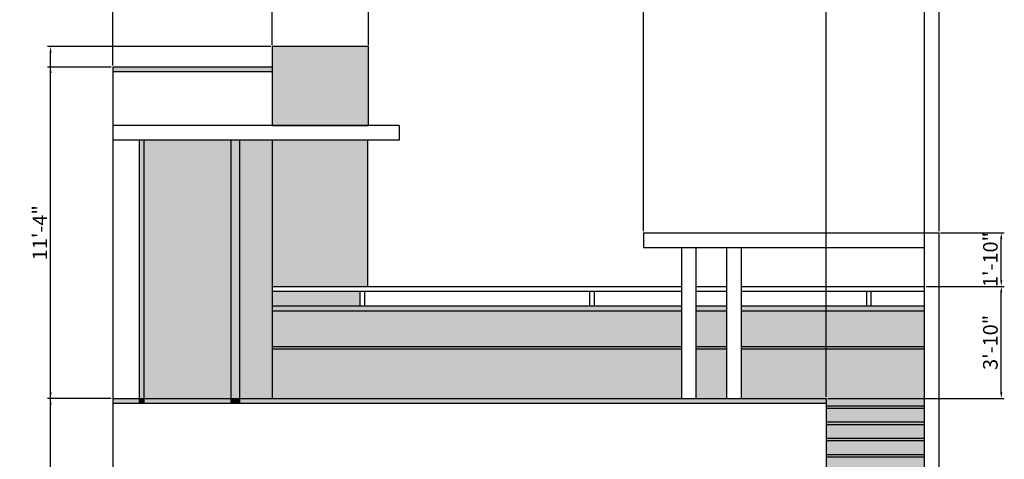
# Model space of a CAD drawing. Units: millimetres. Extents: x 67033 to 68301, y 155969 to 157209.
# Tile 9 of 17: x 67889 to 68293, y 156325 to 156506. Entities that reach past the tile are written whole.
import ezdxf

# ---------------------------------------------------------------- set-up
doc = ezdxf.new("R2010")
doc.units = ezdxf.units.MM
for name, color, linetype, lineweight in [('A-ANNO-DIMS', 2, 'Continuous', 18), ('A-ELEV', 7, 'Continuous', 25), ('A-ELEV-PATT', 252, 'Continuous', 13)]:
    doc.layers.add(name, color=color, linetype=linetype, lineweight=lineweight)
doc.styles.get("Standard").update_dxf_attribs({"font": 'arial.ttf'})
doc.dimstyles.new('ISO-25', dxfattribs={"dimtxt": 6, "dimasz": 2.5, "dimexe": 1.25, "dimexo": 0.625, "dimtad": 1, "dimdec": 0, "dimlunit": 3, "dimtxsty": 'Standard', "dimcen": 2.5, "dimadec": 0, "dimazin": 0, "dimtfac": 1, "dimtdec": 0, "dimtmove": 0, "dimatfit": 3, "dimfxl": 1, "dimarcsym": 0})

# ---------------------------------------------------------------- blocks, each defined once
blk = doc.blocks.new('*D128')
at = {"layer": 'A-ANNO-DIMS', "color": 0, "lineweight": -2, "transparency": 16777216}
for p, q in [((67927.19, 156486.82), (67927.19, 156521.36)), ((68266.19, 156418.82), (68266.19, 156521.36)), ((67929.69, 156520.11), (68263.69, 156520.11))]:
    blk.add_line(p, q, dxfattribs=at)
at = {"layer": 'A-ANNO-DIMS', "color": 0, "transparency": 16777216}
for points in [[(67929.69, 156520.52), (67929.69, 156519.69), (67927.19, 156520.11)], [(68263.69, 156520.52), (68263.69, 156519.69), (68266.19, 156520.11)]]:
    blk.add_solid(points, dxfattribs=at)
at = {"layer": 'Defpoints', "color": 0, "transparency": 16777216}
for p in [(68266.19, 156520.11), (67927.19, 156486.2), (68266.19, 156418.2)]:
    blk.add_point(p, dxfattribs=at)
at = {"layer": 'A-ANNO-DIMS', "color": 0, "transparency": 16777216, "insert": (68096.69, 156523.8), "char_height": 6, "attachment_point": 5}
blk.add_mtext('28\'-3"', dxfattribs=at)
blk = doc.blocks.new('*D138')
at = {"layer": 'A-ANNO-DIMS', "color": 0, "lineweight": -2, "transparency": 16777216}
for p, q in [((67926.57, 156350.2), (67900.44, 156350.2)), ((67901.69, 156208.7), (67901.69, 156347.7)), ((67929.24, 156206.2), (67900.44, 156206.2))]:
    blk.add_line(p, q, dxfattribs=at)
at = {"layer": 'A-ANNO-DIMS', "color": 0, "transparency": 16777216}
for points in [[(67901.27, 156347.7), (67902.11, 156347.7), (67901.69, 156350.2)], [(67901.27, 156208.7), (67902.11, 156208.7), (67901.69, 156206.2)]]:
    blk.add_solid(points, dxfattribs=at)
at = {"layer": 'Defpoints', "color": 0, "transparency": 16777216}
for p in [(67901.69, 156350.2), (67927.19, 156350.2), (67929.86, 156206.2)]:
    blk.add_point(p, dxfattribs=at)
at = {"layer": 'A-ANNO-DIMS', "color": 0, "transparency": 16777216, "insert": (67898, 156278.2), "char_height": 6, "attachment_point": 5, "rotation": 90}
blk.add_mtext('12\'-0"', dxfattribs=at)
blk = doc.blocks.new('*D139')
at = {"layer": 'A-ANNO-DIMS', "color": 0, "lineweight": -2, "transparency": 16777216}
for p, q in [((67926.57, 156486.2), (67900.44, 156486.2)), ((67901.69, 156352.7), (67901.69, 156483.7)), ((67926.57, 156350.2), (67900.44, 156350.2))]:
    blk.add_line(p, q, dxfattribs=at)
at = {"layer": 'A-ANNO-DIMS', "color": 0, "transparency": 16777216}
for points in [[(67901.27, 156483.7), (67902.11, 156483.7), (67901.69, 156486.2)], [(67901.27, 156352.7), (67902.11, 156352.7), (67901.69, 156350.2)]]:
    blk.add_solid(points, dxfattribs=at)
at = {"layer": 'Defpoints', "color": 0, "transparency": 16777216}
for p in [(67901.69, 156486.2), (67927.19, 156486.2), (67927.19, 156350.2)]:
    blk.add_point(p, dxfattribs=at)
at = {"layer": 'A-ANNO-DIMS', "color": 0, "transparency": 16777216, "insert": (67898.05, 156418.2), "char_height": 6, "attachment_point": 5, "rotation": 90}
blk.add_mtext('11\'-4"', dxfattribs=at)
blk = doc.blocks.new('*D140')
at = {"layer": 'A-ANNO-DIMS', "color": 0, "lineweight": -2, "transparency": 16777216}
for p, q in [((67992.02, 156494.61), (67900.44, 156494.61)), ((67901.69, 156002.7), (67901.69, 156492.11)), ((67926.57, 156000.2), (67900.44, 156000.2))]:
    blk.add_line(p, q, dxfattribs=at)
at = {"layer": 'A-ANNO-DIMS', "color": 0, "transparency": 16777216}
for points in [[(67901.27, 156492.11), (67902.11, 156492.11), (67901.69, 156494.61)], [(67901.27, 156002.7), (67902.11, 156002.7), (67901.69, 156000.2)]]:
    blk.add_solid(points, dxfattribs=at)
at = {"layer": 'Defpoints', "color": 0, "transparency": 16777216}
for p in [(67901.69, 156494.61), (67992.65, 156494.61), (67927.19, 156000.2)]:
    blk.add_point(p, dxfattribs=at)
at = {"layer": 'A-ANNO-DIMS', "color": 0, "transparency": 16777216, "insert": (67897.96, 156247.4), "char_height": 6, "attachment_point": 5, "rotation": 90}
blk.add_mtext('41\'-2 1/2"', dxfattribs=at)
blk = doc.blocks.new('*D142')
at = {"layer": 'A-ANNO-DIMS', "color": 0, "lineweight": -2, "transparency": 16777216}
for p, q in [((68260.82, 156396.2), (68292.94, 156396.2)), ((68291.69, 156352.7), (68291.69, 156393.7)), ((68220.53, 156350.2), (68292.94, 156350.2))]:
    blk.add_line(p, q, dxfattribs=at)
at = {"layer": 'A-ANNO-DIMS', "color": 0, "transparency": 16777216}
for points in [[(68291.27, 156393.7), (68292.11, 156393.7), (68291.69, 156396.2)], [(68291.27, 156352.7), (68292.11, 156352.7), (68291.69, 156350.2)]]:
    blk.add_solid(points, dxfattribs=at)
at = {"layer": 'Defpoints', "color": 0, "transparency": 16777216}
for p in [(68260.19, 156396.2), (68291.69, 156396.2), (68219.91, 156350.2)]:
    blk.add_point(p, dxfattribs=at)
at = {"layer": 'A-ANNO-DIMS', "color": 0, "transparency": 16777216, "insert": (68288, 156373.2), "char_height": 6, "attachment_point": 5, "rotation": 90}
blk.add_mtext('3\'-10"', dxfattribs=at)
blk = doc.blocks.new('*D143')
at = {"layer": 'A-ANNO-DIMS', "color": 0, "lineweight": -2, "transparency": 16777216}
for p, q in [((68266.82, 156418.2), (68292.94, 156418.2)), ((68291.69, 156398.7), (68291.69, 156415.7)), ((68260.82, 156396.2), (68292.94, 156396.2))]:
    blk.add_line(p, q, dxfattribs=at)
at = {"layer": 'A-ANNO-DIMS', "color": 0, "transparency": 16777216}
for points in [[(68291.27, 156415.7), (68292.11, 156415.7), (68291.69, 156418.2)], [(68291.27, 156398.7), (68292.11, 156398.7), (68291.69, 156396.2)]]:
    blk.add_solid(points, dxfattribs=at)
at = {"layer": 'Defpoints', "color": 0, "transparency": 16777216}
for p in [(68266.19, 156418.2), (68291.69, 156418.2), (68260.19, 156396.2)]:
    blk.add_point(p, dxfattribs=at)
at = {"layer": 'A-ANNO-DIMS', "color": 0, "transparency": 16777216, "insert": (68288, 156407.2), "char_height": 6, "attachment_point": 5, "rotation": 90}
blk.add_mtext('1\'-10"', dxfattribs=at)
blk = doc.blocks.new('*D144')
at = {"layer": 'A-ANNO-DIMS', "color": 0, "lineweight": -2, "transparency": 16777216}
for p, q in [((67992.65, 156495.23), (67992.65, 156521.36)), ((68032.07, 156495.23), (68032.07, 156521.36)), ((67995.15, 156520.11), (68029.57, 156520.11))]:
    blk.add_line(p, q, dxfattribs=at)
at = {"layer": 'A-ANNO-DIMS', "color": 0, "transparency": 16777216}
for points in [[(67995.15, 156520.52), (67995.15, 156519.69), (67992.65, 156520.11)], [(68029.57, 156520.52), (68029.57, 156519.69), (68032.07, 156520.11)]]:
    blk.add_solid(points, dxfattribs=at)
at = {"layer": 'Defpoints', "color": 0, "transparency": 16777216}
for p in [(68032.07, 156520.11), (67992.65, 156494.61), (68032.07, 156494.61)]:
    blk.add_point(p, dxfattribs=at)
at = {"layer": 'A-ANNO-DIMS', "color": 0, "transparency": 16777216, "insert": (68012.36, 156523.84), "char_height": 6, "attachment_point": 5}
blk.add_mtext('3\'-3 1/2"', dxfattribs=at)
blk = doc.blocks.new('*D145')
at = {"layer": 'A-ANNO-DIMS', "color": 0, "lineweight": -2, "transparency": 16777216}
for p, q in [((68144.87, 156418.82), (68144.87, 156521.36)), ((68266.19, 156418.82), (68266.19, 156521.36)), ((68147.37, 156520.11), (68263.69, 156520.11))]:
    blk.add_line(p, q, dxfattribs=at)
at = {"layer": 'A-ANNO-DIMS', "color": 0, "transparency": 16777216}
for points in [[(68147.37, 156520.52), (68147.37, 156519.69), (68144.87, 156520.11)], [(68263.69, 156520.52), (68263.69, 156519.69), (68266.19, 156520.11)]]:
    blk.add_solid(points, dxfattribs=at)
at = {"layer": 'Defpoints', "color": 0, "transparency": 16777216}
for p in [(68266.19, 156520.11), (68144.87, 156418.2), (68266.19, 156418.2)]:
    blk.add_point(p, dxfattribs=at)
at = {"layer": 'A-ANNO-DIMS', "color": 0, "transparency": 16777216, "insert": (68205.53, 156523.83), "char_height": 6, "attachment_point": 5}
blk.add_mtext('10\'-1 1/2"', dxfattribs=at)
blk = doc.blocks.new('*D146')
at = {"layer": 'A-ANNO-DIMS', "color": 0, "lineweight": -2, "transparency": 16777216}
for p, q in [((68219.91, 156350.82), (68219.91, 156521.36)), ((68260.19, 156396.82), (68260.19, 156521.36)), ((68222.41, 156520.11), (68257.69, 156520.11))]:
    blk.add_line(p, q, dxfattribs=at)
at = {"layer": 'A-ANNO-DIMS', "color": 0, "transparency": 16777216}
for points in [[(68222.41, 156520.52), (68222.41, 156519.69), (68219.91, 156520.11)], [(68257.69, 156520.52), (68257.69, 156519.69), (68260.19, 156520.11)]]:
    blk.add_solid(points, dxfattribs=at)
at = {"layer": 'Defpoints', "color": 0, "transparency": 16777216}
for p in [(68260.19, 156520.11), (68260.19, 156396.2), (68219.91, 156350.2)]:
    blk.add_point(p, dxfattribs=at)
at = {"layer": 'A-ANNO-DIMS', "color": 0, "transparency": 16777216, "insert": (68240.05, 156523.84), "char_height": 6, "attachment_point": 5}
blk.add_mtext('3\'-4 1/2"', dxfattribs=at)

msp = doc.modelspace()

# ---------------------------------------------------------------- hatches: boundary and pattern name
at = {"layer": 'A-ELEV-PATT'}
h = msp.add_hatch(color=256, dxfattribs=at)
h.dxf.hatch_style = 1
h.paths.add_polyline_path([(68032.07, 156494.61), (67992.65, 156494.61), (67992.65, 156462.2), (68032.07, 156462.2)])
h = msp.add_hatch(color=256, dxfattribs=at)
h.dxf.hatch_style = 1
h.paths.add_polyline_path([(67992.65, 156486.2), (67927.19, 156486.2), (67927.19, 156484.2), (67992.65, 156484.2)])
h = msp.add_hatch(color=256, dxfattribs=at)
h.dxf.hatch_style = 1
h.paths.add_polyline_path([(67940.11, 156456.2), (67938.11, 156456.2), (67938.11, 156350.2), (67940.11, 156350.2)])
h = msp.add_hatch(color=256, dxfattribs=at)
h.dxf.hatch_style = 1
h.paths.add_polyline_path([(67975.63, 156456.2), (67940.11, 156456.2), (67940.11, 156350.2), (67975.63, 156350.2)])
h = msp.add_hatch(color=256, dxfattribs=at)
h.dxf.hatch_style = 1
h.paths.add_polyline_path([(67979.14, 156456.2), (67975.63, 156456.2), (67975.63, 156350.2), (67979.14, 156350.2)])
h = msp.add_hatch(color=256, dxfattribs=at)
h.dxf.hatch_style = 1
h.paths.add_polyline_path([(67992.65, 156456.2), (67979.14, 156456.2), (67979.14, 156350.2), (67992.65, 156350.2)])
h = msp.add_hatch(color=256, dxfattribs=at)
h.dxf.hatch_style = 1
h.paths.add_polyline_path([(68031.85, 156456.2), (67992.65, 156456.2), (67992.65, 156396.2), (68031.85, 156396.2)])
h = msp.add_hatch(color=256, dxfattribs=at)
h.dxf.hatch_style = 1
h.paths.add_polyline_path([(68028.58, 156394.2), (67992.65, 156394.2), (67992.65, 156388.2), (68028.58, 156388.2)])
h = msp.add_hatch(color=256, dxfattribs=at)
h.dxf.hatch_style = 1
h.paths.add_polyline_path([(68160.45, 156388.2), (67992.65, 156388.2), (67992.65, 156386.2), (68160.45, 156386.2)])
h = msp.add_hatch(color=256, dxfattribs=at)
h.dxf.hatch_style = 1
h.paths.add_polyline_path([(68178.94, 156388.2), (68166.45, 156388.2), (68166.45, 156386.2), (68178.94, 156386.2)])
h = msp.add_hatch(color=256, dxfattribs=at)
h.dxf.hatch_style = 1
h.paths.add_polyline_path([(68260.19, 156388.2), (68184.94, 156388.2), (68184.94, 156386.2), (68260.19, 156386.2)])
h = msp.add_hatch(color=256, dxfattribs=at)
h.dxf.hatch_style = 1
h.paths.add_polyline_path([(68160.45, 156386.2), (67992.65, 156386.2), (67992.65, 156371.36), (68160.45, 156371.36)])
h = msp.add_hatch(color=256, dxfattribs=at)
h.dxf.hatch_style = 1
h.paths.add_polyline_path([(68178.94, 156386.2), (68166.45, 156386.2), (68166.45, 156371.36), (68178.94, 156371.36)])
h = msp.add_hatch(color=256, dxfattribs=at)
h.dxf.hatch_style = 1
h.paths.add_polyline_path([(68260.19, 156386.2), (68184.94, 156386.2), (68184.94, 156371.36), (68260.19, 156371.36)])
h = msp.add_hatch(color=256, dxfattribs=at)
h.dxf.hatch_style = 1
h.paths.add_polyline_path([(68160.45, 156371.36), (67992.65, 156371.36), (67992.65, 156370.36), (68160.45, 156370.36)])
h = msp.add_hatch(color=256, dxfattribs=at)
h.dxf.hatch_style = 1
h.paths.add_polyline_path([(68178.94, 156371.36), (68166.45, 156371.36), (68166.45, 156370.36), (68178.94, 156370.36)])
h = msp.add_hatch(color=256, dxfattribs=at)
h.dxf.hatch_style = 1
h.paths.add_polyline_path([(68260.19, 156371.36), (68184.94, 156371.36), (68184.94, 156370.36), (68260.19, 156370.36)])
h = msp.add_hatch(color=256, dxfattribs=at)
h.dxf.hatch_style = 1
h.paths.add_polyline_path([(68160.45, 156370.36), (67992.65, 156370.36), (67992.65, 156350.2), (68160.45, 156350.2)])
h = msp.add_hatch(color=256, dxfattribs=at)
h.dxf.hatch_style = 1
h.paths.add_polyline_path([(68178.94, 156370.36), (68166.45, 156370.36), (68166.45, 156350.2), (68178.94, 156350.2)])
h = msp.add_hatch(color=256, dxfattribs=at)
h.dxf.hatch_style = 1
h.paths.add_polyline_path([(68260.19, 156370.36), (68184.94, 156370.36), (68184.94, 156350.2), (68219.91, 156350.2), (68219.91, 156347.23), (68260.19, 156347.23)])
h = msp.add_hatch(color=256, dxfattribs=at)
h.dxf.hatch_style = 1
h.paths.add_polyline_path([(67938.11, 156350.2), (67927.19, 156350.2), (67927.19, 156348.2), (67938.11, 156348.2)])
h = msp.add_hatch(color=256, dxfattribs=at)
h.dxf.hatch_style = 1
h.paths.add_polyline_path([(67940.11, 156350.2), (67938.11, 156350.2), (67938.11, 156348.2), (67940.11, 156348.2)])
h = msp.add_hatch(color=256, dxfattribs=at)
h.dxf.hatch_style = 1
h.paths.add_polyline_path([(67975.63, 156350.2), (67940.11, 156350.2), (67940.11, 156348.2), (67975.63, 156348.2)])
h = msp.add_hatch(color=256, dxfattribs=at)
h.dxf.hatch_style = 1
h.paths.add_polyline_path([(67979.14, 156350.2), (67975.63, 156350.2), (67975.63, 156348.2), (67979.14, 156348.2)])
h = msp.add_hatch(color=256, dxfattribs=at)
h.dxf.hatch_style = 1
h.paths.add_polyline_path([(68219.91, 156350.2), (67979.14, 156350.2), (67979.14, 156348.2), (68219.91, 156348.2)])
h = msp.add_hatch(color=256, dxfattribs=at)
h.dxf.hatch_style = 1
h.paths.add_polyline_path([(68260.19, 156347.23), (68219.91, 156347.23), (68219.91, 156346.23), (68260.19, 156346.23)])
h = msp.add_hatch(color=256, dxfattribs=at)
h.dxf.hatch_style = 1
h.paths.add_polyline_path([(68260.19, 156346.23), (68219.91, 156346.23), (68219.91, 156340.57), (68260.19, 156340.57)])
h = msp.add_hatch(color=256, dxfattribs=at)
h.dxf.hatch_style = 1
h.paths.add_polyline_path([(68260.19, 156340.57), (68219.91, 156340.57), (68219.91, 156339.57), (68260.19, 156339.57)])
h = msp.add_hatch(color=256, dxfattribs=at)
h.dxf.hatch_style = 1
h.paths.add_polyline_path([(68260.19, 156339.57), (68219.91, 156339.57), (68219.91, 156333.91), (68260.19, 156333.91)])
h = msp.add_hatch(color=256, dxfattribs=at)
h.dxf.hatch_style = 1
h.paths.add_polyline_path([(68260.19, 156333.91), (68219.91, 156333.91), (68219.91, 156332.91), (68260.19, 156332.91)])
h = msp.add_hatch(color=256, dxfattribs=at)
h.dxf.hatch_style = 1
h.paths.add_polyline_path([(68260.19, 156332.91), (68219.91, 156332.91), (68219.91, 156327.25), (68260.19, 156327.25)])
h = msp.add_hatch(color=256, dxfattribs=at)
h.dxf.hatch_style = 1
h.paths.add_polyline_path([(68260.19, 156327.25), (68219.91, 156327.25), (68219.91, 156326.25), (68260.19, 156326.25)])
h = msp.add_hatch(color=256, dxfattribs=at)
h.dxf.hatch_style = 1
h.paths.add_polyline_path([(68260.19, 156326.25), (68219.91, 156326.25), (68219.91, 156320.59), (68260.19, 156320.59)])

# ---------------------------------------------------------------- linework, layer by layer
at = {"layer": 'A-ELEV'}
for p, q in [((67927.19, 156486.2), (67927.19, 156000.2)), ((67992.65, 156486.2), (67927.19, 156486.2)), ((67992.65, 156486.2), (67992.65, 156462.2)), ((67992.65, 156484.2), (67927.19, 156484.2)), ((68044.75, 156462.2), (67927.19, 156462.2)), ((68044.75, 156462.2), (68044.75, 156456.2)), ((68044.75, 156456.2), (67927.19, 156456.2)), ((67938.11, 156348.2), (67938.11, 156456.2)), ((67940.11, 156348.2), (67940.11, 156456.2)), ((67975.63, 156456.2), (67975.63, 156348.2)), ((67979.14, 156456.2), (67979.14, 156348.2)), ((67992.65, 156456.2), (67992.65, 156350.2)), ((68031.85, 156396.2), (68031.85, 156456.2)), ((68144.87, 156418.2), (68144.87, 156412.2)), ((68144.87, 156418.2), (68266.19, 156418.2)), ((68266.19, 156000.2), (68266.19, 156418.2)), ((68144.87, 156412.2), (68260.19, 156412.2)), ((68160.45, 156412.2), (68160.45, 156350.2)), ((68166.45, 156412.2), (68166.45, 156350.2)), ((68178.94, 156412.2), (68178.94, 156350.2)), ((68184.94, 156412.2), (68184.94, 156350.2)), ((68260.19, 156169.99), (68260.19, 156412.2)), ((67992.65, 156396.2), (68160.45, 156396.2)), ((68166.45, 156396.2), (68178.94, 156396.2)), ((68184.94, 156396.2), (68260.19, 156396.2)), ((67992.65, 156394.2), (68160.45, 156394.2)), ((68028.58, 156394.2), (68028.58, 156388.2)), ((68030.46, 156394.2), (68030.46, 156388.2)), ((68122.84, 156394.2), (68122.84, 156388.2)), ((68124.72, 156394.2), (68124.72, 156388.2)), ((68166.45, 156394.2), (68178.94, 156394.2)), ((68184.94, 156394.2), (68260.19, 156394.2)), ((68236.36, 156394.2), (68236.36, 156388.2)), ((68238.24, 156394.2), (68238.24, 156388.2)), ((67992.65, 156388.2), (68160.45, 156388.2)), ((68166.45, 156388.2), (68178.94, 156388.2)), ((68184.94, 156388.2), (68260.19, 156388.2)), ((67992.65, 156386.2), (68160.45, 156386.2)), ((68166.45, 156386.2), (68178.94, 156386.2)), ((68184.94, 156386.2), (68260.19, 156386.2)), ((68160.45, 156371.36), (67992.65, 156371.36)), ((68178.94, 156371.36), (68166.45, 156371.36)), ((68260.19, 156371.36), (68184.94, 156371.36)), ((68160.45, 156370.36), (67992.65, 156370.36)), ((68178.94, 156370.36), (68166.45, 156370.36)), ((68260.19, 156370.36), (68184.94, 156370.36)), ((67927.19, 156350.2), (68219.91, 156350.2)), ((67927.19, 156348.2), (68219.91, 156348.2)), ((68219.91, 156350.2), (68219.91, 156180.2)), ((68219.91, 156347.23), (68260.19, 156347.23)), ((68219.91, 156346.23), (68260.19, 156346.23)), ((68219.91, 156340.57), (68260.19, 156340.57)), ((68219.91, 156339.57), (68260.19, 156339.57)), ((68219.91, 156333.91), (68260.19, 156333.91)), ((68219.91, 156332.91), (68260.19, 156332.91)), ((68219.91, 156327.25), (68260.19, 156327.25)), ((68219.91, 156326.25), (68260.19, 156326.25))]:
    msp.add_line(p, q, dxfattribs=at)
msp.add_lwpolyline([(67992.65, 156462.2), (68032.07, 156462.2), (68032.07, 156494.61), (67992.65, 156494.61)], close=True, dxfattribs=at)

# ---------------------------------------------------------------- dimensions: what is measured, and where the dimension line sits
at = {"layer": 'A-ANNO-DIMS'}
for base, p1, p2, picture, middle in [((68032.07, 156520.11), (67992.65, 156494.61), (68032.07, 156494.61), '*D144', (68012.36, 156523.84)), ((68266.19, 156520.11), (68144.87, 156418.2), (68266.19, 156418.2), '*D145', (68205.53, 156523.83)), ((68260.19, 156520.11), (68219.91, 156350.2), (68260.19, 156396.2), '*D146', (68240.05, 156523.84)), ((68266.19, 156520.11), (67927.19, 156486.2), (68266.19, 156418.2), '*D128', (68096.69, 156523.8))]:
    dim = msp.add_linear_dim(base=base, p1=p1, p2=p2, dimstyle='ISO-25', override={"dimdec": 1, "dimlfac": 1, "dimrnd": 0, "dimzin": 1, "dimdsep": 46, "dimlunit": 4, "dimfrac": 2}, dxfattribs=at)
    dim.commit()
    dim.dimension.update_dxf_attribs({"geometry": picture, "text_midpoint": middle})
for base, p1, p2, picture, middle in [((67901.69, 156494.61), (67927.19, 156000.2), (67992.65, 156494.61), '*D140', (67897.96, 156247.4)), ((67901.69, 156486.2), (67927.19, 156350.2), (67927.19, 156486.2), '*D139', (67898.05, 156418.2)), ((68291.69, 156418.2), (68260.19, 156396.2), (68266.19, 156418.2), '*D143', (68288, 156407.2)), ((68291.69, 156396.2), (68219.91, 156350.2), (68260.19, 156396.2), '*D142', (68288, 156373.2)), ((67901.69, 156350.2), (67929.86, 156206.2), (67927.19, 156350.2), '*D138', (67898, 156278.2))]:
    dim = msp.add_linear_dim(base=base, p1=p1, p2=p2, angle=90, dimstyle='ISO-25', override={"dimdec": 1, "dimlfac": 1, "dimrnd": 0, "dimzin": 1, "dimdsep": 46, "dimlunit": 4, "dimfrac": 2}, dxfattribs=at)
    dim.commit()
    dim.dimension.update_dxf_attribs({"geometry": picture, "text_midpoint": middle})

doc.saveas('drawing.dxf')
